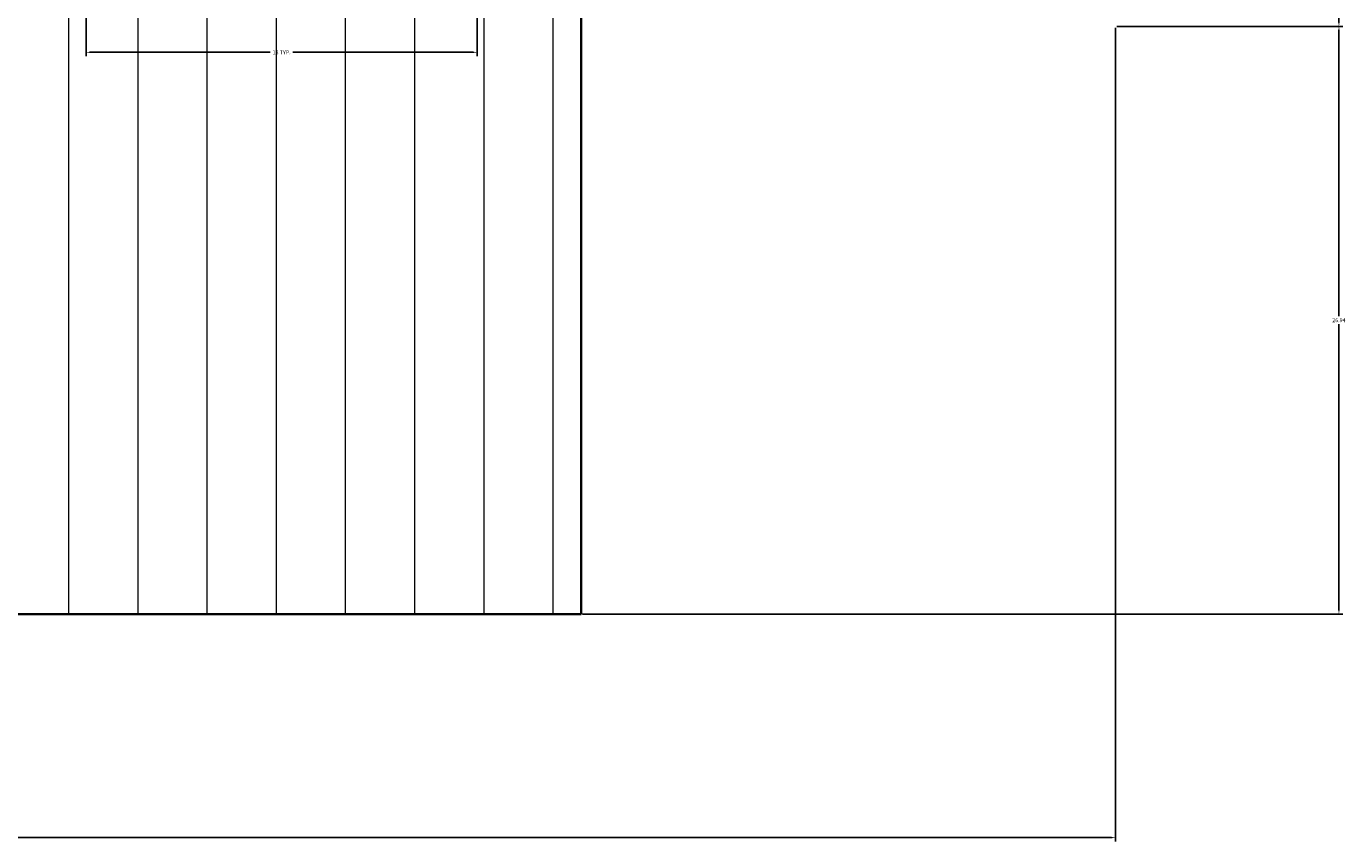
# Model space of a CAD drawing. Units: millimetres. Extents: x 446512 to 447461, y 70395 to 70610.
# Tile 34 of 39: x 447401 to 447461, y 70395 to 70432. Entities that reach past the tile are written whole.
import ezdxf

# ---------------------------------------------------------------- set-up
doc = ezdxf.new("R2010")
doc.units = ezdxf.units.MM
for name, color, linetype, lineweight in [('A-ANNO-DIMS', 2, 'Continuous', 18), ('A-FURN', 7, 'Continuous', 35), ('A-FURN-PATT', 38, 'Continuous', 13)]:
    doc.layers.add(name, color=color, linetype=linetype, lineweight=lineweight)
doc.styles.get("Standard").update_dxf_attribs({"font": 'arial.ttf'})
doc.dimstyles.get("Standard").update_dxf_attribs({"dimtxt": 0.18, "dimasz": 0.18, "dimexe": 0.18, "dimexo": 0.0625, "dimgap": 0.09, "dimtad": 0, "dimtih": 1, "dimtoh": 1, "dimdec": 4, "dimzin": 0, "dimdsep": 46, "dimtxsty": 'Standard', "dimcen": 0.09, "dimadec": 0, "dimazin": 0, "dimtfac": 1, "dimtdec": 4, "dimtofl": 0, "dimtmove": 0, "dimatfit": 3, "dimfxl": 1, "dimtolj": 1, "dimtzin": 0, "dimarcsym": 0})

# ---------------------------------------------------------------- blocks, each defined once
blk = doc.blocks.new('*D6')
at = {"layer": 'A-ANNO-DIMS', "color": 0, "lineweight": -2, "transparency": 16777216}
for p, q in [((447403.306, 70436.225), (447403.306, 70430.885)), ((447421.247, 70436.225), (447421.247, 70430.885)), ((447403.486, 70431.065), (447411.757, 70431.065)), ((447421.067, 70431.065), (447412.796, 70431.065))]:
    blk.add_line(p, q, dxfattribs=at)
at = {"layer": 'A-ANNO-DIMS', "color": 0, "transparency": 16777216}
for points in [[(447403.486, 70431.095), (447403.486, 70431.035), (447403.306, 70431.065)], [(447421.067, 70431.095), (447421.067, 70431.035), (447421.247, 70431.065)]]:
    blk.add_solid(points, dxfattribs=at)
at = {"layer": 'Defpoints', "color": 0, "transparency": 16777216}
for p in [(447403.306, 70436.288), (447421.247, 70436.288), (447421.247, 70431.065)]:
    blk.add_point(p, dxfattribs=at)
at = {"layer": 'A-ANNO-DIMS', "color": 0, "transparency": 16777216, "insert": (447412.276, 70431.065), "char_height": 0.18, "attachment_point": 5}
blk.add_mtext('\\A1;18 TYP.', dxfattribs=at)
blk = doc.blocks.new('*D61')
at = {"layer": 'A-ANNO-DIMS', "color": 0, "lineweight": -2, "transparency": 16777216}
for p, q in [((447254.943, 70452.792), (447254.943, 70394.885)), ((447450.532, 70432.19), (447450.532, 70394.885)), ((447255.123, 70395.065), (447352.352, 70395.065)), ((447450.352, 70395.065), (447353.122, 70395.065))]:
    blk.add_line(p, q, dxfattribs=at)
at = {"layer": 'A-ANNO-DIMS', "color": 0, "transparency": 16777216}
for points in [[(447255.123, 70395.095), (447255.123, 70395.035), (447254.943, 70395.065)], [(447450.352, 70395.095), (447450.352, 70395.035), (447450.532, 70395.065)]]:
    blk.add_solid(points, dxfattribs=at)
at = {"layer": 'Defpoints', "color": 0, "transparency": 16777216}
for p in [(447254.943, 70452.855), (447450.532, 70432.253), (447450.532, 70395.065)]:
    blk.add_point(p, dxfattribs=at)
at = {"layer": 'A-ANNO-DIMS', "color": 0, "transparency": 16777216, "insert": (447352.737, 70395.065), "char_height": 0.18, "attachment_point": 5}
blk.add_mtext('\\A1;195.6', dxfattribs=at)
blk = doc.blocks.new('*D67')
at = {"layer": 'A-ANNO-DIMS', "color": 0, "lineweight": -2, "transparency": 16777216}
for p, q in [((447450.594, 70432.253), (447460.962, 70432.253)), ((447460.782, 70432.073), (447460.782, 70418.965)), ((447460.782, 70405.495), (447460.782, 70418.602)), ((447426.077, 70405.315), (447460.962, 70405.315))]:
    blk.add_line(p, q, dxfattribs=at)
at = {"layer": 'A-ANNO-DIMS', "color": 0, "transparency": 16777216}
for points in [[(447460.752, 70432.073), (447460.812, 70432.073), (447460.782, 70432.253)], [(447460.752, 70405.495), (447460.812, 70405.495), (447460.782, 70405.315)]]:
    blk.add_solid(points, dxfattribs=at)
at = {"layer": 'Defpoints', "color": 0, "transparency": 16777216}
for p in [(447450.532, 70432.253), (447460.782, 70432.253), (447426.014, 70405.315)]:
    blk.add_point(p, dxfattribs=at)
at = {"layer": 'A-ANNO-DIMS', "color": 0, "transparency": 16777216, "insert": (447460.782, 70418.784), "char_height": 0.18, "attachment_point": 5}
blk.add_mtext('\\A1;26.94', dxfattribs=at)
blk = doc.blocks.new('*D68')
at = {"layer": 'A-ANNO-DIMS', "color": 0, "lineweight": -2, "transparency": 16777216}
for p, q in [((447450.594, 70436.288), (447460.962, 70436.288)), ((447460.782, 70436.108), (447460.782, 70434.452)), ((447460.782, 70432.433), (447460.782, 70434.088)), ((447450.594, 70432.253), (447460.962, 70432.253))]:
    blk.add_line(p, q, dxfattribs=at)
at = {"layer": 'A-ANNO-DIMS', "color": 0, "transparency": 16777216}
for points in [[(447460.752, 70436.108), (447460.812, 70436.108), (447460.782, 70436.288)], [(447460.752, 70432.433), (447460.812, 70432.433), (447460.782, 70432.253)]]:
    blk.add_solid(points, dxfattribs=at)
at = {"layer": 'Defpoints', "color": 0, "transparency": 16777216}
for p in [(447450.532, 70436.288), (447460.782, 70436.288), (447450.532, 70432.253)]:
    blk.add_point(p, dxfattribs=at)
at = {"layer": 'A-ANNO-DIMS', "color": 0, "transparency": 16777216, "insert": (447460.782, 70434.27), "char_height": 0.18, "attachment_point": 5}
blk.add_mtext('\\A1;4.035', dxfattribs=at)

msp = doc.modelspace()

# ---------------------------------------------------------------- hatches: boundary and pattern name
at = {"layer": 'A-FURN-PATT'}
h = msp.add_hatch(dxfattribs=at)
h.set_pattern_fill('ANSI31', color=256, angle=45)
h.set_pattern_definition([(90, (127.5626, 0), (-3.175, 0), [])])
h.paths.add_polyline_path([(447426.0142, 70599.7147), (447365.4251, 70599.7147), (447365.4251, 70405.3145), (447426.0142, 70405.3145)])

# ---------------------------------------------------------------- linework, layer by layer
at = {"layer": 'A-FURN'}
for p, q in [((447426.0142, 70405.3145), (447426.0142, 70599.7147)), ((447365.4251, 70405.3145), (447426.0142, 70405.3145))]:
    msp.add_line(p, q, dxfattribs=at)

# ---------------------------------------------------------------- dimensions: what is measured, and where the dimension line sits
at = {"layer": 'A-ANNO-DIMS'}
dim = msp.add_linear_dim(base=(447450.5318, 70395.0645), p1=(447254.9427, 70452.855), p2=(447450.5318, 70432.2526), dimstyle='Standard', override={"dimdec": 1, "dimlfac": 1, "dimrnd": 0, "dimzin": 0, "dimdsep": 46, "dimlunit": 2}, dxfattribs=at)
dim.commit()
dim.dimension.update_dxf_attribs({"geometry": '*D61', "text_midpoint": (447352.7372, 70395.0645)})
dim = msp.add_linear_dim(base=(447421.2469, 70431.0648), p1=(447403.3055, 70436.2876), p2=(447421.2469, 70436.2876), text='<> TYP.', dimstyle='Standard', override={"dimdec": 0, "dimlfac": 1, "dimrnd": 0, "dimzin": 0, "dimdsep": 46, "dimlunit": 2}, dxfattribs=at)
dim.commit()
dim.dimension.update_dxf_attribs({"geometry": '*D6', "text_midpoint": (447412.2762, 70431.0648)})
for base, p1, p2, override, picture, middle in [((447460.7818, 70436.2876), (447450.5318, 70432.2526), (447450.5318, 70436.2876), {"dimdec": 3, "dimlfac": 1, "dimrnd": 0, "dimzin": 0, "dimdsep": 46, "dimlunit": 2}, '*D68', (447460.7818, 70434.2701)), ((447460.7818, 70432.2526), (447426.0142, 70405.3145), (447450.5318, 70432.2526), {"dimdec": 2, "dimlfac": 1, "dimrnd": 0, "dimzin": 0, "dimdsep": 46, "dimlunit": 2}, '*D67', (447460.7818, 70418.7836))]:
    dim = msp.add_linear_dim(base=base, p1=p1, p2=p2, angle=90, dimstyle='Standard', override=override, dxfattribs=at)
    dim.commit()
    dim.dimension.update_dxf_attribs({"geometry": picture, "text_midpoint": middle})

doc.saveas('drawing.dxf')
